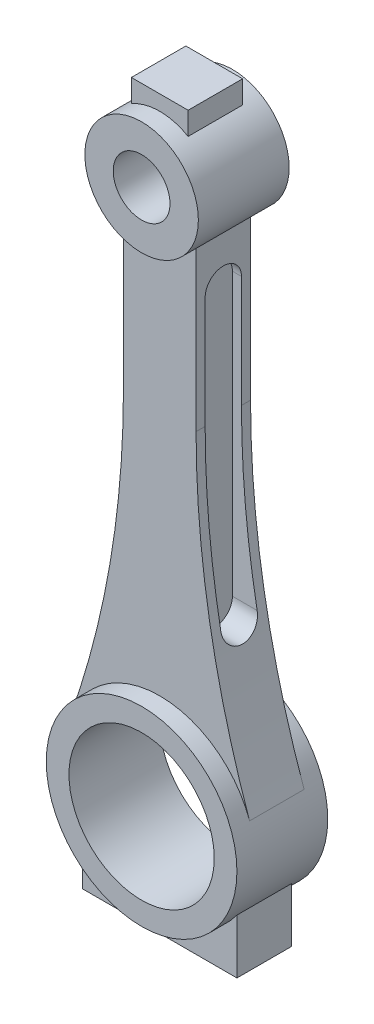
ISO-10303-21;
HEADER;
FILE_DESCRIPTION(('STEP AP214'),'2;1');
FILE_NAME('part.step','',(''),(''),'','','');
FILE_SCHEMA(('AUTOMOTIVE_DESIGN { 1 0 10303 214 1 1 1 1 }'));
ENDSEC;
DATA;
#1=APPLICATION_CONTEXT('core data for automotive mechanical design processes');
#2=APPLICATION_PROTOCOL_DEFINITION('international standard','automotive_design',2000,#1);
#3=PRODUCT_CONTEXT('',#1,'mechanical');
#4=PRODUCT('Part','Part','',(#3));
#5=PRODUCT_RELATED_PRODUCT_CATEGORY('part','',(#4));
#6=PRODUCT_DEFINITION_FORMATION('','',#4);
#7=PRODUCT_DEFINITION_CONTEXT('part definition',#1,'design');
#8=PRODUCT_DEFINITION('design','',#6,#7);
#9=PRODUCT_DEFINITION_SHAPE('','',#8);
#10=(LENGTH_UNIT() NAMED_UNIT(*) SI_UNIT(.MILLI.,.METRE.));
#11=(NAMED_UNIT(*) PLANE_ANGLE_UNIT() SI_UNIT($,.RADIAN.));
#12=(NAMED_UNIT(*) SI_UNIT($,.STERADIAN.) SOLID_ANGLE_UNIT());
#13=UNCERTAINTY_MEASURE_WITH_UNIT(LENGTH_MEASURE(1.E-05),#10,'distance_accuracy_value','');
#14=(GEOMETRIC_REPRESENTATION_CONTEXT(3) GLOBAL_UNCERTAINTY_ASSIGNED_CONTEXT((#13)) GLOBAL_UNIT_ASSIGNED_CONTEXT((#10,
#11,#12)) REPRESENTATION_CONTEXT('',''));
#15=CARTESIAN_POINT('',(0.,0.,0.));
#16=DIRECTION('',(0.,0.,1.));
#17=DIRECTION('',(1.,0.,0.));
#18=AXIS2_PLACEMENT_3D('',#15,#16,#17);
#19=CARTESIAN_POINT('',(212.132819979024,75.3953136438508,6.));
#20=DIRECTION('',(0.,0.,-1.));
#21=DIRECTION('',(-1.,0.,0.));
#22=AXIS2_PLACEMENT_3D('',#19,#20,#21);
#23=CYLINDRICAL_SURFACE('',#22,204.132819979024);
#24=CARTESIAN_POINT('',(11.4544735884215,38.,-4.00000000000001));
#25=CARTESIAN_POINT('',(11.4757515518411,37.8858086335559,-4.00000967356236));
#26=CARTESIAN_POINT('',(11.497127848932,37.7716411229782,-3.9951101211208));
#27=CARTESIAN_POINT('',(11.5399210356049,37.544152772884,-3.97557755361704));
#28=CARTESIAN_POINT('',(11.5613379239584,37.4308319082382,-3.9609448286138));
#29=CARTESIAN_POINT('',(11.6040518019029,37.2058589467753,-3.92203609087538));
#30=CARTESIAN_POINT('',(11.6253488219803,37.0942064124742,-3.89776265395078));
#31=CARTESIAN_POINT('',(11.6676599337569,36.8733657612217,-3.83975872762631));
#32=CARTESIAN_POINT('',(11.688674029376,36.7641776101131,-3.80602836938937));
#33=CARTESIAN_POINT('',(11.7510730473326,36.4413470108117,-3.69089420326938));
#34=CARTESIAN_POINT('',(11.7918289081029,36.2323636826891,-3.59553432969807));
#35=CARTESIAN_POINT('',(11.8702126062764,35.833491871712,-3.37027556179513));
#36=CARTESIAN_POINT('',(11.9078413597511,35.643597793309,-3.24038682968163));
#37=CARTESIAN_POINT('',(11.9784728244352,35.2894796680367,-2.950436910244));
#38=CARTESIAN_POINT('',(12.0115036519544,35.1250988255321,-2.79057453802655));
#39=CARTESIAN_POINT('',(12.0720036427705,34.8256035029566,-2.44449926104123));
#40=CARTESIAN_POINT('',(12.0994724370193,34.6904909648341,-2.25828460915733));
#41=CARTESIAN_POINT('',(12.1473413477104,34.4559602912754,-1.86832249559897));
#42=CARTESIAN_POINT('',(12.1678582991115,34.3559510460777,-1.66494499104501));
#43=CARTESIAN_POINT('',(12.201667760202,34.1915558050773,-1.24372237948287));
#44=CARTESIAN_POINT('',(12.2149615713728,34.1271633917176,-1.02587988675161));
#45=CARTESIAN_POINT('',(12.2336033492388,34.0369591960168,-0.586274812122705));
#46=CARTESIAN_POINT('',(12.2390950212482,34.0104496060439,-0.364661335561854));
#47=CARTESIAN_POINT('',(12.2423732155319,33.9946184843632,0.0799443502249422));
#48=CARTESIAN_POINT('',(12.2401601145853,34.0052951341723,0.302936491499035));
#49=CARTESIAN_POINT('',(12.2281765408432,34.0632127244266,0.741781925824315));
#50=CARTESIAN_POINT('',(12.2184766498272,34.1101121767816,0.957682365575702));
#51=CARTESIAN_POINT('',(12.1919895794175,34.2385791029979,1.37844153266758));
#52=CARTESIAN_POINT('',(12.1752023313576,34.3201469127454,1.58330015300714));
#53=CARTESIAN_POINT('',(12.1350793834177,34.5159552856904,1.977397761575));
#54=CARTESIAN_POINT('',(12.1117098081663,34.6303649264094,2.16654921549123));
#55=CARTESIAN_POINT('',(12.0593260749273,34.8882465100265,2.52297125984127));
#56=CARTESIAN_POINT('',(12.0303117725959,35.0317191961119,2.69024129055298));
#57=CARTESIAN_POINT('',(11.9671383735568,35.3461665633751,3.00114206510914));
#58=CARTESIAN_POINT('',(11.9329025496515,35.5175545383741,3.14433904981939));
#59=CARTESIAN_POINT('',(11.8607975408038,35.8812712267655,3.40006280722765));
#60=CARTESIAN_POINT('',(11.8229268395298,36.0736086840292,3.51257670427656));
#61=CARTESIAN_POINT('',(11.744011046999,36.4777513253325,3.70593438635491));
#62=CARTESIAN_POINT('',(11.7029182624971,36.6898643551292,3.78611370956408));
#63=CARTESIAN_POINT('',(11.619535719839,37.1241795414682,3.90944320644274));
#64=CARTESIAN_POINT('',(11.5772477716993,37.3463667203578,3.95264656840455));
#65=CARTESIAN_POINT('',(11.5215540274852,37.6417241762258,3.98457340087694));
#66=CARTESIAN_POINT('',(11.5080944382148,37.713314753212,3.99036111817268));
#67=CARTESIAN_POINT('',(11.4812368188341,37.8565916807734,3.99806924003837));
#68=CARTESIAN_POINT('',(11.467838723541,37.9282776734255,3.99999606757804));
#69=CARTESIAN_POINT('',(11.4544735884215,38.,3.99999999999999));
#70=B_SPLINE_CURVE_WITH_KNOTS('',3,(#24,#25,#26,#27,#28,#29,#30,#31,#32,#33,#34,#35,#36,#37,#38,
#39,#40,#41,#42,#43,#44,#45,#46,#47,#48,#49,#50,#51,#52,#53,#54,#55,#56,#57,#58,#59,#60,#61,#62,
#63,#64,#65,#66,#67,#68,#69),.UNSPECIFIED.,.F.,.F.,(4,2,2,2,2,2,2,2,2,2,2,2,2,2,2,2,2,2,2,2,2,2,
4),(0.,0.348357600629775,0.69670482029576,1.04495903090802,1.39320841164155,2.08947857427321,
2.78554404346984,3.47714614167073,4.1687941135383,4.84816302804556,5.52740949173436,
6.19397531687089,6.86050854603356,7.52083364695975,8.18116514562694,8.84495910470898,
9.50877004017901,10.1834922182609,10.8584970981523,11.546741507572,12.2339942357506,
12.4531452672714,12.6719314158043),.UNSPECIFIED.);
#71=CARTESIAN_POINT('',(11.4544735884215,38.,-4.00000000000001));
#72=VERTEX_POINT('',#71);
#73=CARTESIAN_POINT('',(11.4544735884215,38.,3.99999999999999));
#74=VERTEX_POINT('',#73);
#75=EDGE_CURVE('E406',#72,#74,#70,.T.);
#76=ORIENTED_EDGE('',*,*,#75,.T.);
#77=CARTESIAN_POINT('',(212.132819979024,75.3953136438508,4.));
#78=DIRECTION('',(0.,0.,-1.));
#79=DIRECTION('',(0.,1.,0.));
#80=AXIS2_PLACEMENT_3D('',#77,#78,#79);
#81=CIRCLE('',#80,204.132819979024);
#82=CARTESIAN_POINT('',(8.,75.3953136438507,4.));
#83=VERTEX_POINT('',#82);
#84=EDGE_CURVE('E265',#74,#83,#81,.T.);
#85=ORIENTED_EDGE('',*,*,#84,.T.);
#86=DIRECTION('',(0.,0.,-1.));
#87=VECTOR('',#86,1.);
#88=CARTESIAN_POINT('',(8.,75.3953136438507,6.));
#89=LINE('',#88,#87);
#90=CARTESIAN_POINT('',(8.,75.3953136438507,6.));
#91=VERTEX_POINT('',#90);
#92=EDGE_CURVE('E386',#91,#83,#89,.T.);
#93=ORIENTED_EDGE('',*,*,#92,.F.);
#94=CARTESIAN_POINT('',(212.132819979024,75.3953136438508,6.));
#95=DIRECTION('',(0.,0.,1.));
#96=DIRECTION('',(1.,0.,0.));
#97=AXIS2_PLACEMENT_3D('',#94,#95,#96);
#98=CIRCLE('',#97,204.132819979024);
#99=CARTESIAN_POINT('',(19.7873824881444,7.03274443356765,6.));
#100=VERTEX_POINT('',#99);
#101=EDGE_CURVE('E341',#91,#100,#98,.T.);
#102=ORIENTED_EDGE('',*,*,#101,.T.);
#103=DIRECTION('',(0.,0.,-1.));
#104=VECTOR('',#103,1.);
#105=CARTESIAN_POINT('',(19.7873824881444,7.03274443356765,6.));
#106=LINE('',#105,#104);
#107=CARTESIAN_POINT('',(19.7873824881444,7.03274443356765,-6.));
#108=VERTEX_POINT('',#107);
#109=EDGE_CURVE('E357',#100,#108,#106,.T.);
#110=ORIENTED_EDGE('',*,*,#109,.T.);
#111=CARTESIAN_POINT('',(212.132819979024,75.3953136438508,-6.));
#112=DIRECTION('',(0.,0.,1.));
#113=DIRECTION('',(1.,0.,0.));
#114=AXIS2_PLACEMENT_3D('',#111,#112,#113);
#115=CIRCLE('',#114,204.132819979024);
#116=CARTESIAN_POINT('',(8.,75.3953136438507,-6.));
#117=VERTEX_POINT('',#116);
#118=EDGE_CURVE('E338',#117,#108,#115,.T.);
#119=ORIENTED_EDGE('',*,*,#118,.F.);
#120=CARTESIAN_POINT('',(8.,75.3953136438507,-4.));
#121=VERTEX_POINT('',#120);
#122=EDGE_CURVE('E389',#121,#117,#89,.T.);
#123=ORIENTED_EDGE('',*,*,#122,.F.);
#124=CARTESIAN_POINT('',(212.132819979024,75.3953136438508,-4.00000000000001));
#125=DIRECTION('',(0.,0.,1.));
#126=DIRECTION('',(0.,-1.,0.));
#127=AXIS2_PLACEMENT_3D('',#124,#125,#126);
#128=CIRCLE('',#127,204.132819979024);
#129=EDGE_CURVE('E67',#121,#72,#128,.T.);
#130=ORIENTED_EDGE('',*,*,#129,.T.);
#131=EDGE_LOOP('',(#76,#85,#93,#102,#110,#119,#123,#130));
#132=FACE_BOUND('',#131,.T.);
#133=ADVANCED_FACE('F44',(#132),#23,.F.);
#134=CARTESIAN_POINT('',(8.00000000000002,0.,6.));
#135=DIRECTION('',(-1.,0.,0.));
#136=DIRECTION('',(0.,-1.,0.));
#137=AXIS2_PLACEMENT_3D('',#134,#135,#136);
#138=PLANE('',#137);
#139=DIRECTION('',(0.,-1.,0.));
#140=VECTOR('',#139,1.);
#141=CARTESIAN_POINT('',(8.00000000000002,0.,3.99999999999999));
#142=LINE('',#141,#140);
#143=CARTESIAN_POINT('',(8.00000000000001,100.,4.));
#144=VERTEX_POINT('',#143);
#145=EDGE_CURVE('E407',#144,#83,#142,.T.);
#146=ORIENTED_EDGE('',*,*,#145,.F.);
#147=CARTESIAN_POINT('',(8.,100.,0.));
#148=DIRECTION('',(-1.,0.,0.));
#149=DIRECTION('',(0.,-1.,0.));
#150=AXIS2_PLACEMENT_3D('',#147,#148,#149);
#151=CIRCLE('',#150,4.);
#152=CARTESIAN_POINT('',(8.00000000000001,100.,-4.));
#153=VERTEX_POINT('',#152);
#154=EDGE_CURVE('E408',#153,#144,#151,.F.);
#155=ORIENTED_EDGE('',*,*,#154,.F.);
#156=DIRECTION('',(0.,1.,0.));
#157=VECTOR('',#156,1.);
#158=CARTESIAN_POINT('',(8.00000000000002,0.,-4.00000000000001));
#159=LINE('',#158,#157);
#160=EDGE_CURVE('E399',#121,#153,#159,.T.);
#161=ORIENTED_EDGE('',*,*,#160,.F.);
#162=ORIENTED_EDGE('',*,*,#122,.T.);
#163=DIRECTION('',(0.,1.,0.));
#164=VECTOR('',#163,1.);
#165=CARTESIAN_POINT('',(8.00000000000002,0.,-6.));
#166=LINE('',#165,#164);
#167=CARTESIAN_POINT('',(8.,110.395313643851,-6.));
#168=VERTEX_POINT('',#167);
#169=EDGE_CURVE('E363',#117,#168,#166,.T.);
#170=ORIENTED_EDGE('',*,*,#169,.T.);
#171=DIRECTION('',(0.,0.,-1.));
#172=VECTOR('',#171,1.);
#173=CARTESIAN_POINT('',(8.,110.395313643851,6.));
#174=LINE('',#173,#172);
#175=CARTESIAN_POINT('',(8.,110.395313643851,6.));
#176=VERTEX_POINT('',#175);
#177=EDGE_CURVE('E387',#176,#168,#174,.T.);
#178=ORIENTED_EDGE('',*,*,#177,.F.);
#179=DIRECTION('',(0.,1.,0.));
#180=VECTOR('',#179,1.);
#181=CARTESIAN_POINT('',(8.00000000000002,0.,6.));
#182=LINE('',#181,#180);
#183=EDGE_CURVE('E343',#91,#176,#182,.T.);
#184=ORIENTED_EDGE('',*,*,#183,.F.);
#185=ORIENTED_EDGE('',*,*,#92,.T.);
#186=EDGE_LOOP('',(#146,#155,#161,#162,#170,#178,#184,#185));
#187=FACE_BOUND('',#186,.T.);
#188=ADVANCED_FACE('F536',(#187),#138,.F.);
#189=CARTESIAN_POINT('',(0.,120.,10.));
#190=DIRECTION('',(0.,0.,-1.));
#191=DIRECTION('',(-1.,0.,0.));
#192=AXIS2_PLACEMENT_3D('',#189,#190,#191);
#193=CYLINDRICAL_SURFACE('',#192,6.25);
#194=CARTESIAN_POINT('',(0.,120.,10.));
#195=DIRECTION('',(0.,0.,1.));
#196=DIRECTION('',(1.,0.,0.));
#197=AXIS2_PLACEMENT_3D('',#194,#195,#196);
#198=CIRCLE('',#197,6.25);
#199=CARTESIAN_POINT('',(6.25,120.,10.));
#200=VERTEX_POINT('',#199);
#201=EDGE_CURVE('E392',#200,#200,#198,.T.);
#202=ORIENTED_EDGE('',*,*,#201,.T.);
#203=EDGE_LOOP('',(#202));
#204=FACE_BOUND('',#203,.T.);
#205=CARTESIAN_POINT('',(0.,120.,-10.));
#206=DIRECTION('',(0.,0.,1.));
#207=DIRECTION('',(1.,0.,0.));
#208=AXIS2_PLACEMENT_3D('',#205,#206,#207);
#209=CIRCLE('',#208,6.25);
#210=CARTESIAN_POINT('',(6.25,120.,-10.));
#211=VERTEX_POINT('',#210);
#212=EDGE_CURVE('E394',#211,#211,#209,.T.);
#213=ORIENTED_EDGE('',*,*,#212,.F.);
#214=EDGE_LOOP('',(#213));
#215=FACE_BOUND('',#214,.T.);
#216=ADVANCED_FACE('F50',(#204,#215),#193,.F.);
#217=CARTESIAN_POINT('',(0.,120.,10.));
#218=DIRECTION('',(0.,0.,-1.));
#219=DIRECTION('',(-1.,0.,0.));
#220=AXIS2_PLACEMENT_3D('',#217,#218,#219);
#221=CYLINDRICAL_SURFACE('',#220,12.5);
#222=DIRECTION('',(0.,0.,-1.));
#223=VECTOR('',#222,1.);
#224=CARTESIAN_POINT('',(6.25,130.825317547305,6.));
#225=LINE('',#224,#223);
#226=CARTESIAN_POINT('',(6.25,130.825317547305,6.));
#227=VERTEX_POINT('',#226);
#228=CARTESIAN_POINT('',(6.25,130.825317547305,-6.));
#229=VERTEX_POINT('',#228);
#230=EDGE_CURVE('E324',#227,#229,#225,.T.);
#231=ORIENTED_EDGE('',*,*,#230,.F.);
#232=CARTESIAN_POINT('',(0.,120.,6.));
#233=DIRECTION('',(0.,0.,1.));
#234=DIRECTION('',(1.,0.,0.));
#235=AXIS2_PLACEMENT_3D('',#232,#233,#234);
#236=CIRCLE('',#235,12.5);
#237=CARTESIAN_POINT('',(-6.25,130.825317547305,6.));
#238=VERTEX_POINT('',#237);
#239=EDGE_CURVE('E297',#227,#238,#236,.T.);
#240=ORIENTED_EDGE('',*,*,#239,.T.);
#241=DIRECTION('',(0.,0.,-1.));
#242=VECTOR('',#241,1.);
#243=CARTESIAN_POINT('',(-6.25,130.825317547305,6.));
#244=LINE('',#243,#242);
#245=CARTESIAN_POINT('',(-6.25,130.825317547305,-6.));
#246=VERTEX_POINT('',#245);
#247=EDGE_CURVE('E310',#238,#246,#244,.T.);
#248=ORIENTED_EDGE('',*,*,#247,.T.);
#249=CARTESIAN_POINT('',(0.,120.,-6.));
#250=DIRECTION('',(0.,0.,1.));
#251=DIRECTION('',(1.,0.,0.));
#252=AXIS2_PLACEMENT_3D('',#249,#250,#251);
#253=CIRCLE('',#252,12.5);
#254=EDGE_CURVE('E299',#229,#246,#253,.T.);
#255=ORIENTED_EDGE('',*,*,#254,.F.);
#256=EDGE_LOOP('',(#231,#240,#248,#255));
#257=FACE_BOUND('',#256,.T.);
#258=DIRECTION('',(0.,0.,-1.));
#259=VECTOR('',#258,1.);
#260=CARTESIAN_POINT('',(-7.99999999999999,110.395313643851,6.));
#261=LINE('',#260,#259);
#262=CARTESIAN_POINT('',(-7.99999999999999,110.395313643851,6.));
#263=VERTEX_POINT('',#262);
#264=CARTESIAN_POINT('',(-7.99999999999999,110.395313643851,-6.));
#265=VERTEX_POINT('',#264);
#266=EDGE_CURVE('E382',#263,#265,#261,.T.);
#267=ORIENTED_EDGE('',*,*,#266,.F.);
#268=CARTESIAN_POINT('',(0.,120.,6.));
#269=DIRECTION('',(0.,0.,1.));
#270=DIRECTION('',(1.,0.,0.));
#271=AXIS2_PLACEMENT_3D('',#268,#269,#270);
#272=CIRCLE('',#271,12.5);
#273=EDGE_CURVE('E346',#263,#176,#272,.T.);
#274=ORIENTED_EDGE('',*,*,#273,.T.);
#275=ORIENTED_EDGE('',*,*,#177,.T.);
#276=CARTESIAN_POINT('',(0.,120.,-6.));
#277=DIRECTION('',(0.,0.,1.));
#278=DIRECTION('',(1.,0.,0.));
#279=AXIS2_PLACEMENT_3D('',#276,#277,#278);
#280=CIRCLE('',#279,12.5);
#281=EDGE_CURVE('E365',#265,#168,#280,.T.);
#282=ORIENTED_EDGE('',*,*,#281,.F.);
#283=EDGE_LOOP('',(#267,#274,#275,#282));
#284=FACE_BOUND('',#283,.T.);
#285=CARTESIAN_POINT('',(0.,120.,10.));
#286=DIRECTION('',(0.,0.,1.));
#287=DIRECTION('',(1.,0.,0.));
#288=AXIS2_PLACEMENT_3D('',#285,#286,#287);
#289=CIRCLE('',#288,12.5);
#290=CARTESIAN_POINT('',(12.5,120.,10.));
#291=VERTEX_POINT('',#290);
#292=EDGE_CURVE('E396',#291,#291,#289,.T.);
#293=ORIENTED_EDGE('',*,*,#292,.F.);
#294=EDGE_LOOP('',(#293));
#295=FACE_BOUND('',#294,.T.);
#296=CARTESIAN_POINT('',(0.,120.,-10.));
#297=DIRECTION('',(0.,0.,1.));
#298=DIRECTION('',(1.,0.,0.));
#299=AXIS2_PLACEMENT_3D('',#296,#297,#298);
#300=CIRCLE('',#299,12.5);
#301=CARTESIAN_POINT('',(12.5,120.,-10.));
#302=VERTEX_POINT('',#301);
#303=EDGE_CURVE('E400',#302,#302,#300,.T.);
#304=ORIENTED_EDGE('',*,*,#303,.T.);
#305=EDGE_LOOP('',(#304));
#306=FACE_BOUND('',#305,.T.);
#307=ADVANCED_FACE('F567',(#257,#284,#295,#306),#221,.T.);
#308=CARTESIAN_POINT('',(0.,0.,10.));
#309=DIRECTION('',(0.,0.,1.));
#310=DIRECTION('',(1.,0.,0.));
#311=AXIS2_PLACEMENT_3D('',#308,#309,#310);
#312=PLANE('',#311);
#313=ORIENTED_EDGE('',*,*,#201,.F.);
#314=EDGE_LOOP('',(#313));
#315=FACE_BOUND('',#314,.T.);
#316=ORIENTED_EDGE('',*,*,#292,.T.);
#317=EDGE_LOOP('',(#316));
#318=FACE_BOUND('',#317,.T.);
#319=ADVANCED_FACE('F648',(#315,#318),#312,.T.);
#320=CARTESIAN_POINT('',(0.,0.,-10.));
#321=DIRECTION('',(0.,0.,1.));
#322=DIRECTION('',(1.,0.,0.));
#323=AXIS2_PLACEMENT_3D('',#320,#321,#322);
#324=PLANE('',#323);
#325=ORIENTED_EDGE('',*,*,#212,.T.);
#326=EDGE_LOOP('',(#325));
#327=FACE_BOUND('',#326,.T.);
#328=ORIENTED_EDGE('',*,*,#303,.F.);
#329=EDGE_LOOP('',(#328));
#330=FACE_BOUND('',#329,.T.);
#331=ADVANCED_FACE('F620',(#327,#330),#324,.F.);
#332=CARTESIAN_POINT('',(-7.99999999999999,0.,6.));
#333=DIRECTION('',(-1.,0.,0.));
#334=DIRECTION('',(0.,0.,1.));
#335=AXIS2_PLACEMENT_3D('',#332,#333,#334);
#336=PLANE('',#335);
#337=DIRECTION('',(0.,-1.,0.));
#338=VECTOR('',#337,1.);
#339=CARTESIAN_POINT('',(-7.99999999999999,0.,-4.00000000000001));
#340=LINE('',#339,#338);
#341=CARTESIAN_POINT('',(-8.,100.,-4.));
#342=VERTEX_POINT('',#341);
#343=CARTESIAN_POINT('',(-8.00000000000001,75.3953136438507,-4.00000000000001));
#344=VERTEX_POINT('',#343);
#345=EDGE_CURVE('E239',#342,#344,#340,.T.);
#346=ORIENTED_EDGE('',*,*,#345,.F.);
#347=CARTESIAN_POINT('',(-7.99999999999999,100.,0.));
#348=DIRECTION('',(-1.,0.,0.));
#349=DIRECTION('',(0.,0.,1.));
#350=AXIS2_PLACEMENT_3D('',#347,#348,#349);
#351=CIRCLE('',#350,4.);
#352=CARTESIAN_POINT('',(-8.,100.,4.));
#353=VERTEX_POINT('',#352);
#354=EDGE_CURVE('E11',#353,#342,#351,.T.);
#355=ORIENTED_EDGE('',*,*,#354,.F.);
#356=DIRECTION('',(0.,1.,0.));
#357=VECTOR('',#356,1.);
#358=CARTESIAN_POINT('',(-7.99999999999999,0.,3.99999999999999));
#359=LINE('',#358,#357);
#360=CARTESIAN_POINT('',(-8.00000000000001,75.3953136438507,4.));
#361=VERTEX_POINT('',#360);
#362=EDGE_CURVE('E216',#361,#353,#359,.T.);
#363=ORIENTED_EDGE('',*,*,#362,.F.);
#364=DIRECTION('',(0.,0.,-1.));
#365=VECTOR('',#364,1.);
#366=CARTESIAN_POINT('',(-7.99999999999999,75.3953136438507,6.));
#367=LINE('',#366,#365);
#368=CARTESIAN_POINT('',(-7.99999999999999,75.3953136438507,6.));
#369=VERTEX_POINT('',#368);
#370=EDGE_CURVE('E379',#369,#361,#367,.T.);
#371=ORIENTED_EDGE('',*,*,#370,.F.);
#372=DIRECTION('',(0.,1.,0.));
#373=VECTOR('',#372,1.);
#374=CARTESIAN_POINT('',(-7.99999999999999,0.,6.));
#375=LINE('',#374,#373);
#376=EDGE_CURVE('E348',#369,#263,#375,.T.);
#377=ORIENTED_EDGE('',*,*,#376,.T.);
#378=ORIENTED_EDGE('',*,*,#266,.T.);
#379=DIRECTION('',(0.,1.,0.));
#380=VECTOR('',#379,1.);
#381=CARTESIAN_POINT('',(-7.99999999999999,0.,-6.));
#382=LINE('',#381,#380);
#383=CARTESIAN_POINT('',(-7.99999999999999,75.3953136438507,-6.));
#384=VERTEX_POINT('',#383);
#385=EDGE_CURVE('E370',#384,#265,#382,.T.);
#386=ORIENTED_EDGE('',*,*,#385,.F.);
#387=EDGE_CURVE('E377',#344,#384,#367,.T.);
#388=ORIENTED_EDGE('',*,*,#387,.F.);
#389=EDGE_LOOP('',(#346,#355,#363,#371,#377,#378,#386,#388));
#390=FACE_BOUND('',#389,.T.);
#391=ADVANCED_FACE('F507',(#390),#336,.T.);
#392=CARTESIAN_POINT('',(-212.132819979024,75.3953136438507,6.));
#393=DIRECTION('',(0.,0.,-1.));
#394=DIRECTION('',(-1.,0.,0.));
#395=AXIS2_PLACEMENT_3D('',#392,#393,#394);
#396=CYLINDRICAL_SURFACE('',#395,204.132819979024);
#397=CARTESIAN_POINT('',(-11.4544735884215,38.,3.99999999999999));
#398=CARTESIAN_POINT('',(-11.4757515518411,37.8858086335559,4.00000967356234));
#399=CARTESIAN_POINT('',(-11.497127848932,37.7716411229782,3.99511012112078));
#400=CARTESIAN_POINT('',(-11.5399210356049,37.544152772884,3.97557755361703));
#401=CARTESIAN_POINT('',(-11.5613379239584,37.4308319082382,3.96094482861378));
#402=CARTESIAN_POINT('',(-11.6040518019029,37.2058589467753,3.92203609087537));
#403=CARTESIAN_POINT('',(-11.6253488219802,37.0942064124742,3.89776265395076));
#404=CARTESIAN_POINT('',(-11.6676599337569,36.8733657612217,3.83975872762629));
#405=CARTESIAN_POINT('',(-11.6886740293759,36.7641776101131,3.80602836938935));
#406=CARTESIAN_POINT('',(-11.7510730473326,36.4413470108117,3.69089420326937));
#407=CARTESIAN_POINT('',(-11.7918289081029,36.2323636826891,3.59553432969806));
#408=CARTESIAN_POINT('',(-11.8702126062764,35.833491871712,3.37027556179512));
#409=CARTESIAN_POINT('',(-11.9078413597511,35.643597793309,3.24038682968162));
#410=CARTESIAN_POINT('',(-11.9784728244352,35.2894796680367,2.95043691024399));
#411=CARTESIAN_POINT('',(-12.0115036519544,35.1250988255321,2.79057453802654));
#412=CARTESIAN_POINT('',(-12.0720036427705,34.8256035029566,2.44449926104123));
#413=CARTESIAN_POINT('',(-12.0994724370193,34.6904909648341,2.25828460915732));
#414=CARTESIAN_POINT('',(-12.1473413477104,34.4559602912754,1.86832249559895));
#415=CARTESIAN_POINT('',(-12.1678582991115,34.3559510460777,1.66494499104499));
#416=CARTESIAN_POINT('',(-12.201667760202,34.1915558050773,1.24372237948286));
#417=CARTESIAN_POINT('',(-12.2149615713728,34.1271633917176,1.02587988675159));
#418=CARTESIAN_POINT('',(-12.2336033492388,34.0369591960168,0.586274812122689));
#419=CARTESIAN_POINT('',(-12.2390950212481,34.0104496060439,0.364661335561839));
#420=CARTESIAN_POINT('',(-12.2423732155318,33.9946184843632,-0.0799443502249572));
#421=CARTESIAN_POINT('',(-12.2401601145853,34.0052951341723,-0.30293649149905));
#422=CARTESIAN_POINT('',(-12.2281765408432,34.0632127244266,-0.74178192582433));
#423=CARTESIAN_POINT('',(-12.2184766498272,34.1101121767816,-0.957682365575717));
#424=CARTESIAN_POINT('',(-12.1919895794175,34.2385791029979,-1.3784415326676));
#425=CARTESIAN_POINT('',(-12.1752023313576,34.3201469127454,-1.58330015300716));
#426=CARTESIAN_POINT('',(-12.1350793834177,34.5159552856904,-1.97739776157502));
#427=CARTESIAN_POINT('',(-12.1117098081663,34.6303649264094,-2.16654921549125));
#428=CARTESIAN_POINT('',(-12.0593260749273,34.8882465100265,-2.52297125984129));
#429=CARTESIAN_POINT('',(-12.0303117725959,35.0317191961119,-2.690241290553));
#430=CARTESIAN_POINT('',(-11.9671383735568,35.3461665633751,-3.00114206510916));
#431=CARTESIAN_POINT('',(-11.9329025496515,35.5175545383741,-3.14433904981941));
#432=CARTESIAN_POINT('',(-11.8607975408038,35.8812712267655,-3.40006280722766));
#433=CARTESIAN_POINT('',(-11.8229268395298,36.0736086840292,-3.51257670427658));
#434=CARTESIAN_POINT('',(-11.744011046999,36.4777513253325,-3.70593438635493));
#435=CARTESIAN_POINT('',(-11.7029182624971,36.6898643551292,-3.78611370956409));
#436=CARTESIAN_POINT('',(-11.6195357198389,37.1241795414682,-3.90944320644275));
#437=CARTESIAN_POINT('',(-11.5772477716993,37.3463667203578,-3.95264656840456));
#438=CARTESIAN_POINT('',(-11.5215540274853,37.6417241762258,-3.98457340087696));
#439=CARTESIAN_POINT('',(-11.5080944382149,37.713314753212,-3.9903611181727));
#440=CARTESIAN_POINT('',(-11.4812368188341,37.8565916807733,-3.99806924003838));
#441=CARTESIAN_POINT('',(-11.467838723541,37.9282776734255,-3.99999606757806));
#442=CARTESIAN_POINT('',(-11.4544735884215,38.,-4.00000000000001));
#443=B_SPLINE_CURVE_WITH_KNOTS('',3,(#397,#398,#399,#400,#401,#402,#403,#404,#405,#406,#407,
#408,#409,#410,#411,#412,#413,#414,#415,#416,#417,#418,#419,#420,#421,#422,#423,#424,#425,#426,
#427,#428,#429,#430,#431,#432,#433,#434,#435,#436,#437,#438,#439,#440,#441,#442),.UNSPECIFIED.,
.F.,.F.,(4,2,2,2,2,2,2,2,2,2,2,2,2,2,2,2,2,2,2,2,2,2,4),(0.,0.348357600629778,0.696704820295753,
1.044959030908,1.39320841164154,2.0894785742732,2.78554404346983,3.47714614167072,
4.1687941135383,4.84816302804556,5.52740949173436,6.19397531687089,6.86050854603355,
7.52083364695974,8.18116514562693,8.84495910470897,9.508770040179,10.1834922182609,
10.8584970981523,11.546741507572,12.2339942357505,12.4531452672714,12.6719314158043),.UNSPECIFIED.);
#444=CARTESIAN_POINT('',(-11.4544735884215,38.,3.99999999999999));
#445=VERTEX_POINT('',#444);
#446=CARTESIAN_POINT('',(-11.4544735884215,38.,-4.00000000000001));
#447=VERTEX_POINT('',#446);
#448=EDGE_CURVE('E509',#445,#447,#443,.T.);
#449=ORIENTED_EDGE('',*,*,#448,.T.);
#450=CARTESIAN_POINT('',(-212.132819979024,75.3953136438507,-4.00000000000001));
#451=DIRECTION('',(0.,0.,-1.));
#452=DIRECTION('',(0.,1.,0.));
#453=AXIS2_PLACEMENT_3D('',#450,#451,#452);
#454=CIRCLE('',#453,204.132819979024);
#455=EDGE_CURVE('E52',#447,#344,#454,.F.);
#456=ORIENTED_EDGE('',*,*,#455,.T.);
#457=ORIENTED_EDGE('',*,*,#387,.T.);
#458=CARTESIAN_POINT('',(-212.132819979024,75.3953136438507,-6.));
#459=DIRECTION('',(0.,0.,1.));
#460=DIRECTION('',(1.,0.,0.));
#461=AXIS2_PLACEMENT_3D('',#458,#459,#460);
#462=CIRCLE('',#461,204.132819979024);
#463=CARTESIAN_POINT('',(-19.7873824881444,7.03274443356764,-6.));
#464=VERTEX_POINT('',#463);
#465=EDGE_CURVE('E367',#384,#464,#462,.F.);
#466=ORIENTED_EDGE('',*,*,#465,.T.);
#467=DIRECTION('',(0.,0.,-1.));
#468=VECTOR('',#467,1.);
#469=CARTESIAN_POINT('',(-19.7873824881444,7.03274443356764,6.));
#470=LINE('',#469,#468);
#471=CARTESIAN_POINT('',(-19.7873824881444,7.03274443356764,6.));
#472=VERTEX_POINT('',#471);
#473=EDGE_CURVE('E380',#472,#464,#470,.T.);
#474=ORIENTED_EDGE('',*,*,#473,.F.);
#475=CARTESIAN_POINT('',(-212.132819979024,75.3953136438507,6.));
#476=DIRECTION('',(0.,0.,1.));
#477=DIRECTION('',(1.,0.,0.));
#478=AXIS2_PLACEMENT_3D('',#475,#476,#477);
#479=CIRCLE('',#478,204.132819979024);
#480=EDGE_CURVE('E352',#369,#472,#479,.F.);
#481=ORIENTED_EDGE('',*,*,#480,.F.);
#482=ORIENTED_EDGE('',*,*,#370,.T.);
#483=CARTESIAN_POINT('',(-212.132819979024,75.3953136438507,4.));
#484=DIRECTION('',(0.,0.,1.));
#485=DIRECTION('',(0.,-1.,0.));
#486=AXIS2_PLACEMENT_3D('',#483,#484,#485);
#487=CIRCLE('',#486,204.132819979024);
#488=EDGE_CURVE('E420',#361,#445,#487,.F.);
#489=ORIENTED_EDGE('',*,*,#488,.T.);
#490=EDGE_LOOP('',(#449,#456,#457,#466,#474,#481,#482,#489));
#491=FACE_BOUND('',#490,.T.);
#492=ADVANCED_FACE('F498',(#491),#396,.F.);
#493=CARTESIAN_POINT('',(0.,0.,6.));
#494=DIRECTION('',(0.,0.,1.));
#495=DIRECTION('',(1.,0.,0.));
#496=AXIS2_PLACEMENT_3D('',#493,#494,#495);
#497=PLANE('',#496);
#498=ORIENTED_EDGE('',*,*,#101,.F.);
#499=ORIENTED_EDGE('',*,*,#183,.T.);
#500=ORIENTED_EDGE('',*,*,#273,.F.);
#501=ORIENTED_EDGE('',*,*,#376,.F.);
#502=ORIENTED_EDGE('',*,*,#480,.T.);
#503=CARTESIAN_POINT('',(0.,0.,6.));
#504=DIRECTION('',(0.,0.,1.));
#505=DIRECTION('',(1.,0.,0.));
#506=AXIS2_PLACEMENT_3D('',#503,#504,#505);
#507=CIRCLE('',#506,21.);
#508=EDGE_CURVE('E356',#100,#472,#507,.T.);
#509=ORIENTED_EDGE('',*,*,#508,.F.);
#510=EDGE_LOOP('',(#498,#499,#500,#501,#502,#509));
#511=FACE_BOUND('',#510,.T.);
#512=ADVANCED_FACE('F500',(#511),#497,.T.);
#513=CARTESIAN_POINT('',(0.,0.,-6.));
#514=DIRECTION('',(0.,0.,1.));
#515=DIRECTION('',(1.,0.,0.));
#516=AXIS2_PLACEMENT_3D('',#513,#514,#515);
#517=PLANE('',#516);
#518=ORIENTED_EDGE('',*,*,#118,.T.);
#519=CARTESIAN_POINT('',(0.,0.,-6.));
#520=DIRECTION('',(0.,0.,1.));
#521=DIRECTION('',(1.,0.,0.));
#522=AXIS2_PLACEMENT_3D('',#519,#520,#521);
#523=CIRCLE('',#522,21.);
#524=EDGE_CURVE('E344',#108,#464,#523,.T.);
#525=ORIENTED_EDGE('',*,*,#524,.T.);
#526=ORIENTED_EDGE('',*,*,#465,.F.);
#527=ORIENTED_EDGE('',*,*,#385,.T.);
#528=ORIENTED_EDGE('',*,*,#281,.T.);
#529=ORIENTED_EDGE('',*,*,#169,.F.);
#530=EDGE_LOOP('',(#518,#525,#526,#527,#528,#529));
#531=FACE_BOUND('',#530,.T.);
#532=ADVANCED_FACE('F494',(#531),#517,.F.);
#533=CARTESIAN_POINT('',(0.,0.,10.));
#534=DIRECTION('',(0.,0.,-1.));
#535=DIRECTION('',(-1.,0.,0.));
#536=AXIS2_PLACEMENT_3D('',#533,#534,#535);
#537=CYLINDRICAL_SURFACE('',#536,16.);
#538=CARTESIAN_POINT('',(0.,0.,10.));
#539=DIRECTION('',(0.,0.,1.));
#540=DIRECTION('',(1.,0.,0.));
#541=AXIS2_PLACEMENT_3D('',#538,#539,#540);
#542=CIRCLE('',#541,16.);
#543=CARTESIAN_POINT('',(16.,0.,10.));
#544=VERTEX_POINT('',#543);
#545=EDGE_CURVE('E328',#544,#544,#542,.T.);
#546=ORIENTED_EDGE('',*,*,#545,.T.);
#547=EDGE_LOOP('',(#546));
#548=FACE_BOUND('',#547,.T.);
#549=CARTESIAN_POINT('',(0.,0.,-10.));
#550=DIRECTION('',(0.,0.,1.));
#551=DIRECTION('',(1.,0.,0.));
#552=AXIS2_PLACEMENT_3D('',#549,#550,#551);
#553=CIRCLE('',#552,16.);
#554=CARTESIAN_POINT('',(16.,0.,-10.));
#555=VERTEX_POINT('',#554);
#556=EDGE_CURVE('E327',#555,#555,#553,.T.);
#557=ORIENTED_EDGE('',*,*,#556,.F.);
#558=EDGE_LOOP('',(#557));
#559=FACE_BOUND('',#558,.T.);
#560=ADVANCED_FACE('F491',(#548,#559),#537,.F.);
#561=CARTESIAN_POINT('',(0.,0.,10.));
#562=DIRECTION('',(0.,0.,-1.));
#563=DIRECTION('',(-1.,0.,0.));
#564=AXIS2_PLACEMENT_3D('',#561,#562,#563);
#565=CYLINDRICAL_SURFACE('',#564,21.);
#566=DIRECTION('',(0.,0.,-1.));
#567=VECTOR('',#566,1.);
#568=CARTESIAN_POINT('',(-17.,-12.328828005938,6.));
#569=LINE('',#568,#567);
#570=CARTESIAN_POINT('',(-17.,-12.328828005938,6.));
#571=VERTEX_POINT('',#570);
#572=CARTESIAN_POINT('',(-17.,-12.328828005938,-6.));
#573=VERTEX_POINT('',#572);
#574=EDGE_CURVE('E294',#571,#573,#569,.T.);
#575=ORIENTED_EDGE('',*,*,#574,.F.);
#576=CARTESIAN_POINT('',(0.,0.,6.));
#577=DIRECTION('',(0.,0.,1.));
#578=DIRECTION('',(1.,0.,0.));
#579=AXIS2_PLACEMENT_3D('',#576,#577,#578);
#580=CIRCLE('',#579,21.);
#581=CARTESIAN_POINT('',(17.,-12.328828005938,6.));
#582=VERTEX_POINT('',#581);
#583=EDGE_CURVE('E266',#571,#582,#580,.T.);
#584=ORIENTED_EDGE('',*,*,#583,.T.);
#585=DIRECTION('',(0.,0.,-1.));
#586=VECTOR('',#585,1.);
#587=CARTESIAN_POINT('',(17.,-12.328828005938,6.));
#588=LINE('',#587,#586);
#589=CARTESIAN_POINT('',(17.,-12.328828005938,-6.));
#590=VERTEX_POINT('',#589);
#591=EDGE_CURVE('E279',#582,#590,#588,.T.);
#592=ORIENTED_EDGE('',*,*,#591,.T.);
#593=CARTESIAN_POINT('',(0.,0.,-6.));
#594=DIRECTION('',(0.,0.,1.));
#595=DIRECTION('',(1.,0.,0.));
#596=AXIS2_PLACEMENT_3D('',#593,#594,#595);
#597=CIRCLE('',#596,21.);
#598=EDGE_CURVE('E264',#573,#590,#597,.T.);
#599=ORIENTED_EDGE('',*,*,#598,.F.);
#600=EDGE_LOOP('',(#575,#584,#592,#599));
#601=FACE_BOUND('',#600,.T.);
#602=ORIENTED_EDGE('',*,*,#508,.T.);
#603=ORIENTED_EDGE('',*,*,#473,.T.);
#604=ORIENTED_EDGE('',*,*,#524,.F.);
#605=ORIENTED_EDGE('',*,*,#109,.F.);
#606=EDGE_LOOP('',(#602,#603,#604,#605));
#607=FACE_BOUND('',#606,.T.);
#608=CARTESIAN_POINT('',(0.,0.,10.));
#609=DIRECTION('',(0.,0.,1.));
#610=DIRECTION('',(1.,0.,0.));
#611=AXIS2_PLACEMENT_3D('',#608,#609,#610);
#612=CIRCLE('',#611,21.);
#613=CARTESIAN_POINT('',(21.,0.,10.));
#614=VERTEX_POINT('',#613);
#615=EDGE_CURVE('E335',#614,#614,#612,.T.);
#616=ORIENTED_EDGE('',*,*,#615,.F.);
#617=EDGE_LOOP('',(#616));
#618=FACE_BOUND('',#617,.T.);
#619=CARTESIAN_POINT('',(0.,0.,-10.));
#620=DIRECTION('',(0.,0.,1.));
#621=DIRECTION('',(1.,0.,0.));
#622=AXIS2_PLACEMENT_3D('',#619,#620,#621);
#623=CIRCLE('',#622,21.);
#624=CARTESIAN_POINT('',(21.,0.,-10.));
#625=VERTEX_POINT('',#624);
#626=EDGE_CURVE('E334',#625,#625,#623,.T.);
#627=ORIENTED_EDGE('',*,*,#626,.T.);
#628=EDGE_LOOP('',(#627));
#629=FACE_BOUND('',#628,.T.);
#630=ADVANCED_FACE('F482',(#601,#607,#618,#629),#565,.T.);
#631=CARTESIAN_POINT('',(0.,0.,10.));
#632=DIRECTION('',(0.,0.,1.));
#633=DIRECTION('',(1.,0.,0.));
#634=AXIS2_PLACEMENT_3D('',#631,#632,#633);
#635=PLANE('',#634);
#636=ORIENTED_EDGE('',*,*,#545,.F.);
#637=EDGE_LOOP('',(#636));
#638=FACE_BOUND('',#637,.T.);
#639=ORIENTED_EDGE('',*,*,#615,.T.);
#640=EDGE_LOOP('',(#639));
#641=FACE_BOUND('',#640,.T.);
#642=ADVANCED_FACE('F481',(#638,#641),#635,.T.);
#643=CARTESIAN_POINT('',(0.,0.,-10.));
#644=DIRECTION('',(0.,0.,1.));
#645=DIRECTION('',(1.,0.,0.));
#646=AXIS2_PLACEMENT_3D('',#643,#644,#645);
#647=PLANE('',#646);
#648=ORIENTED_EDGE('',*,*,#556,.T.);
#649=EDGE_LOOP('',(#648));
#650=FACE_BOUND('',#649,.T.);
#651=ORIENTED_EDGE('',*,*,#626,.F.);
#652=EDGE_LOOP('',(#651));
#653=FACE_BOUND('',#652,.T.);
#654=ADVANCED_FACE('F479',(#650,#653),#647,.F.);
#655=CARTESIAN_POINT('',(6.24999999999995,0.,6.));
#656=DIRECTION('',(1.,0.,0.));
#657=DIRECTION('',(0.,1.,0.));
#658=AXIS2_PLACEMENT_3D('',#655,#656,#657);
#659=PLANE('',#658);
#660=DIRECTION('',(0.,-1.,0.));
#661=VECTOR('',#660,1.);
#662=CARTESIAN_POINT('',(6.24999999999995,0.,-6.));
#663=LINE('',#662,#661);
#664=CARTESIAN_POINT('',(6.25,135.825317547305,-6.));
#665=VERTEX_POINT('',#664);
#666=EDGE_CURVE('E315',#665,#229,#663,.T.);
#667=ORIENTED_EDGE('',*,*,#666,.F.);
#668=DIRECTION('',(0.,0.,-1.));
#669=VECTOR('',#668,1.);
#670=CARTESIAN_POINT('',(6.25,135.825317547305,6.));
#671=LINE('',#670,#669);
#672=CARTESIAN_POINT('',(6.25,135.825317547305,6.));
#673=VERTEX_POINT('',#672);
#674=EDGE_CURVE('E323',#673,#665,#671,.T.);
#675=ORIENTED_EDGE('',*,*,#674,.F.);
#676=DIRECTION('',(0.,-1.,0.));
#677=VECTOR('',#676,1.);
#678=CARTESIAN_POINT('',(6.24999999999995,0.,6.));
#679=LINE('',#678,#677);
#680=EDGE_CURVE('E296',#673,#227,#679,.T.);
#681=ORIENTED_EDGE('',*,*,#680,.T.);
#682=ORIENTED_EDGE('',*,*,#230,.T.);
#683=EDGE_LOOP('',(#667,#675,#681,#682));
#684=FACE_BOUND('',#683,.T.);
#685=ADVANCED_FACE('F474',(#684),#659,.T.);
#686=CARTESIAN_POINT('',(0.,135.825317547305,6.));
#687=DIRECTION('',(0.,-1.,0.));
#688=DIRECTION('',(0.,0.,-1.));
#689=AXIS2_PLACEMENT_3D('',#686,#687,#688);
#690=PLANE('',#689);
#691=DIRECTION('',(-1.,0.,0.));
#692=VECTOR('',#691,1.);
#693=CARTESIAN_POINT('',(0.,135.825317547305,-6.));
#694=LINE('',#693,#692);
#695=CARTESIAN_POINT('',(-6.25,135.825317547305,-6.));
#696=VERTEX_POINT('',#695);
#697=EDGE_CURVE('E312',#665,#696,#694,.T.);
#698=ORIENTED_EDGE('',*,*,#697,.T.);
#699=DIRECTION('',(0.,0.,-1.));
#700=VECTOR('',#699,1.);
#701=CARTESIAN_POINT('',(-6.25,135.825317547305,6.));
#702=LINE('',#701,#700);
#703=CARTESIAN_POINT('',(-6.25,135.825317547305,6.));
#704=VERTEX_POINT('',#703);
#705=EDGE_CURVE('E319',#704,#696,#702,.T.);
#706=ORIENTED_EDGE('',*,*,#705,.F.);
#707=DIRECTION('',(-1.,0.,0.));
#708=VECTOR('',#707,1.);
#709=CARTESIAN_POINT('',(0.,135.825317547305,6.));
#710=LINE('',#709,#708);
#711=EDGE_CURVE('E303',#673,#704,#710,.T.);
#712=ORIENTED_EDGE('',*,*,#711,.F.);
#713=ORIENTED_EDGE('',*,*,#674,.T.);
#714=EDGE_LOOP('',(#698,#706,#712,#713));
#715=FACE_BOUND('',#714,.T.);
#716=ADVANCED_FACE('F473',(#715),#690,.F.);
#717=CARTESIAN_POINT('',(-6.25,0.,6.));
#718=DIRECTION('',(1.,0.,0.));
#719=DIRECTION('',(0.,0.,-1.));
#720=AXIS2_PLACEMENT_3D('',#717,#718,#719);
#721=PLANE('',#720);
#722=DIRECTION('',(0.,-1.,0.));
#723=VECTOR('',#722,1.);
#724=CARTESIAN_POINT('',(-6.25,0.,-6.));
#725=LINE('',#724,#723);
#726=EDGE_CURVE('E301',#696,#246,#725,.T.);
#727=ORIENTED_EDGE('',*,*,#726,.T.);
#728=ORIENTED_EDGE('',*,*,#247,.F.);
#729=DIRECTION('',(0.,-1.,0.));
#730=VECTOR('',#729,1.);
#731=CARTESIAN_POINT('',(-6.25,0.,6.));
#732=LINE('',#731,#730);
#733=EDGE_CURVE('E308',#704,#238,#732,.T.);
#734=ORIENTED_EDGE('',*,*,#733,.F.);
#735=ORIENTED_EDGE('',*,*,#705,.T.);
#736=EDGE_LOOP('',(#727,#728,#734,#735));
#737=FACE_BOUND('',#736,.T.);
#738=ADVANCED_FACE('F465',(#737),#721,.F.);
#739=CARTESIAN_POINT('',(0.,0.,6.));
#740=DIRECTION('',(0.,0.,1.));
#741=DIRECTION('',(1.,0.,0.));
#742=AXIS2_PLACEMENT_3D('',#739,#740,#741);
#743=PLANE('',#742);
#744=ORIENTED_EDGE('',*,*,#239,.F.);
#745=ORIENTED_EDGE('',*,*,#680,.F.);
#746=ORIENTED_EDGE('',*,*,#711,.T.);
#747=ORIENTED_EDGE('',*,*,#733,.T.);
#748=EDGE_LOOP('',(#744,#745,#746,#747));
#749=FACE_BOUND('',#748,.T.);
#750=ADVANCED_FACE('F463',(#749),#743,.T.);
#751=CARTESIAN_POINT('',(0.,0.,-6.));
#752=DIRECTION('',(0.,0.,1.));
#753=DIRECTION('',(1.,0.,0.));
#754=AXIS2_PLACEMENT_3D('',#751,#752,#753);
#755=PLANE('',#754);
#756=ORIENTED_EDGE('',*,*,#254,.T.);
#757=ORIENTED_EDGE('',*,*,#726,.F.);
#758=ORIENTED_EDGE('',*,*,#697,.F.);
#759=ORIENTED_EDGE('',*,*,#666,.T.);
#760=EDGE_LOOP('',(#756,#757,#758,#759));
#761=FACE_BOUND('',#760,.T.);
#762=ADVANCED_FACE('F459',(#761),#755,.F.);
#763=CARTESIAN_POINT('',(-17.,0.,6.));
#764=DIRECTION('',(-1.,0.,0.));
#765=DIRECTION('',(0.,-1.,0.));
#766=AXIS2_PLACEMENT_3D('',#763,#764,#765);
#767=PLANE('',#766);
#768=DIRECTION('',(0.,1.,0.));
#769=VECTOR('',#768,1.);
#770=CARTESIAN_POINT('',(-17.,0.,-6.));
#771=LINE('',#770,#769);
#772=CARTESIAN_POINT('',(-17.,-24.328828005938,-6.));
#773=VERTEX_POINT('',#772);
#774=EDGE_CURVE('E283',#773,#573,#771,.T.);
#775=ORIENTED_EDGE('',*,*,#774,.F.);
#776=DIRECTION('',(0.,0.,-1.));
#777=VECTOR('',#776,1.);
#778=CARTESIAN_POINT('',(-17.,-24.328828005938,6.));
#779=LINE('',#778,#777);
#780=CARTESIAN_POINT('',(-17.,-24.328828005938,6.));
#781=VERTEX_POINT('',#780);
#782=EDGE_CURVE('E295',#781,#773,#779,.T.);
#783=ORIENTED_EDGE('',*,*,#782,.F.);
#784=DIRECTION('',(0.,1.,0.));
#785=VECTOR('',#784,1.);
#786=CARTESIAN_POINT('',(-17.,0.,6.));
#787=LINE('',#786,#785);
#788=EDGE_CURVE('E268',#781,#571,#787,.T.);
#789=ORIENTED_EDGE('',*,*,#788,.T.);
#790=ORIENTED_EDGE('',*,*,#574,.T.);
#791=EDGE_LOOP('',(#775,#783,#789,#790));
#792=FACE_BOUND('',#791,.T.);
#793=ADVANCED_FACE('F454',(#792),#767,.T.);
#794=CARTESIAN_POINT('',(0.,-24.328828005938,6.));
#795=DIRECTION('',(0.,-1.,0.));
#796=DIRECTION('',(1.,0.,0.));
#797=AXIS2_PLACEMENT_3D('',#794,#795,#796);
#798=PLANE('',#797);
#799=DIRECTION('',(-1.,0.,0.));
#800=VECTOR('',#799,1.);
#801=CARTESIAN_POINT('',(0.,-24.328828005938,-6.));
#802=LINE('',#801,#800);
#803=CARTESIAN_POINT('',(17.,-24.328828005938,-6.));
#804=VERTEX_POINT('',#803);
#805=EDGE_CURVE('E285',#804,#773,#802,.T.);
#806=ORIENTED_EDGE('',*,*,#805,.F.);
#807=DIRECTION('',(0.,0.,-1.));
#808=VECTOR('',#807,1.);
#809=CARTESIAN_POINT('',(17.,-24.328828005938,6.));
#810=LINE('',#809,#808);
#811=CARTESIAN_POINT('',(17.,-24.328828005938,6.));
#812=VERTEX_POINT('',#811);
#813=EDGE_CURVE('E289',#812,#804,#810,.T.);
#814=ORIENTED_EDGE('',*,*,#813,.F.);
#815=DIRECTION('',(-1.,0.,0.));
#816=VECTOR('',#815,1.);
#817=CARTESIAN_POINT('',(0.,-24.328828005938,6.));
#818=LINE('',#817,#816);
#819=EDGE_CURVE('E275',#812,#781,#818,.T.);
#820=ORIENTED_EDGE('',*,*,#819,.T.);
#821=ORIENTED_EDGE('',*,*,#782,.T.);
#822=EDGE_LOOP('',(#806,#814,#820,#821));
#823=FACE_BOUND('',#822,.T.);
#824=ADVANCED_FACE('F451',(#823),#798,.T.);
#825=CARTESIAN_POINT('',(17.,0.,6.));
#826=DIRECTION('',(-1.,0.,0.));
#827=DIRECTION('',(0.,-1.,0.));
#828=AXIS2_PLACEMENT_3D('',#825,#826,#827);
#829=PLANE('',#828);
#830=DIRECTION('',(0.,1.,0.));
#831=VECTOR('',#830,1.);
#832=CARTESIAN_POINT('',(17.,0.,-6.));
#833=LINE('',#832,#831);
#834=EDGE_CURVE('E267',#804,#590,#833,.T.);
#835=ORIENTED_EDGE('',*,*,#834,.T.);
#836=ORIENTED_EDGE('',*,*,#591,.F.);
#837=DIRECTION('',(0.,1.,0.));
#838=VECTOR('',#837,1.);
#839=CARTESIAN_POINT('',(17.,0.,6.));
#840=LINE('',#839,#838);
#841=EDGE_CURVE('E274',#812,#582,#840,.T.);
#842=ORIENTED_EDGE('',*,*,#841,.F.);
#843=ORIENTED_EDGE('',*,*,#813,.T.);
#844=EDGE_LOOP('',(#835,#836,#842,#843));
#845=FACE_BOUND('',#844,.T.);
#846=ADVANCED_FACE('F441',(#845),#829,.F.);
#847=CARTESIAN_POINT('',(0.,0.,6.));
#848=DIRECTION('',(0.,0.,1.));
#849=DIRECTION('',(1.,0.,0.));
#850=AXIS2_PLACEMENT_3D('',#847,#848,#849);
#851=PLANE('',#850);
#852=ORIENTED_EDGE('',*,*,#583,.F.);
#853=ORIENTED_EDGE('',*,*,#788,.F.);
#854=ORIENTED_EDGE('',*,*,#819,.F.);
#855=ORIENTED_EDGE('',*,*,#841,.T.);
#856=EDGE_LOOP('',(#852,#853,#854,#855));
#857=FACE_BOUND('',#856,.T.);
#858=ADVANCED_FACE('F442',(#857),#851,.T.);
#859=CARTESIAN_POINT('',(0.,0.,-6.));
#860=DIRECTION('',(0.,0.,1.));
#861=DIRECTION('',(1.,0.,0.));
#862=AXIS2_PLACEMENT_3D('',#859,#860,#861);
#863=PLANE('',#862);
#864=ORIENTED_EDGE('',*,*,#598,.T.);
#865=ORIENTED_EDGE('',*,*,#834,.F.);
#866=ORIENTED_EDGE('',*,*,#805,.T.);
#867=ORIENTED_EDGE('',*,*,#774,.T.);
#868=EDGE_LOOP('',(#864,#865,#866,#867));
#869=FACE_BOUND('',#868,.T.);
#870=ADVANCED_FACE('F438',(#869),#863,.F.);
#871=CARTESIAN_POINT('',(21.,100.,0.));
#872=DIRECTION('',(-1.,0.,0.));
#873=DIRECTION('',(0.,0.,1.));
#874=AXIS2_PLACEMENT_3D('',#871,#872,#873);
#875=CYLINDRICAL_SURFACE('',#874,4.);
#876=ORIENTED_EDGE('',*,*,#154,.T.);
#877=DIRECTION('',(-1.,0.,0.));
#878=VECTOR('',#877,1.);
#879=CARTESIAN_POINT('',(21.,100.,4.));
#880=LINE('',#879,#878);
#881=CARTESIAN_POINT('',(6.,100.,4.));
#882=VERTEX_POINT('',#881);
#883=EDGE_CURVE('E259',#144,#882,#880,.T.);
#884=ORIENTED_EDGE('',*,*,#883,.T.);
#885=CARTESIAN_POINT('',(6.,100.,0.));
#886=DIRECTION('',(1.,0.,0.));
#887=DIRECTION('',(0.,0.,-1.));
#888=AXIS2_PLACEMENT_3D('',#885,#886,#887);
#889=CIRCLE('',#888,4.);
#890=CARTESIAN_POINT('',(6.,100.,-4.));
#891=VERTEX_POINT('',#890);
#892=EDGE_CURVE('E243',#891,#882,#889,.T.);
#893=ORIENTED_EDGE('',*,*,#892,.F.);
#894=DIRECTION('',(-1.,0.,0.));
#895=VECTOR('',#894,1.);
#896=CARTESIAN_POINT('',(21.,100.,-4.));
#897=LINE('',#896,#895);
#898=EDGE_CURVE('E251',#153,#891,#897,.T.);
#899=ORIENTED_EDGE('',*,*,#898,.F.);
#900=EDGE_LOOP('',(#876,#884,#893,#899));
#901=FACE_BOUND('',#900,.T.);
#902=ADVANCED_FACE('F434',(#901),#875,.F.);
#903=CARTESIAN_POINT('',(21.,100.,4.));
#904=DIRECTION('',(0.,0.,-1.));
#905=DIRECTION('',(0.,1.,0.));
#906=AXIS2_PLACEMENT_3D('',#903,#904,#905);
#907=PLANE('',#906);
#908=DIRECTION('',(-1.,0.,0.));
#909=VECTOR('',#908,1.);
#910=CARTESIAN_POINT('',(21.,38.,3.99999999999999));
#911=LINE('',#910,#909);
#912=CARTESIAN_POINT('',(6.,38.,3.99999999999999));
#913=VERTEX_POINT('',#912);
#914=EDGE_CURVE('E260',#74,#913,#911,.T.);
#915=ORIENTED_EDGE('',*,*,#914,.T.);
#916=DIRECTION('',(0.,-1.,0.));
#917=VECTOR('',#916,1.);
#918=CARTESIAN_POINT('',(6.,100.,4.));
#919=LINE('',#918,#917);
#920=EDGE_CURVE('E245',#882,#913,#919,.T.);
#921=ORIENTED_EDGE('',*,*,#920,.F.);
#922=ORIENTED_EDGE('',*,*,#883,.F.);
#923=ORIENTED_EDGE('',*,*,#145,.T.);
#924=ORIENTED_EDGE('',*,*,#84,.F.);
#925=EDGE_LOOP('',(#915,#921,#922,#923,#924));
#926=FACE_BOUND('',#925,.T.);
#927=ADVANCED_FACE('F429',(#926),#907,.T.);
#928=CARTESIAN_POINT('',(21.,38.,0.));
#929=DIRECTION('',(-1.,0.,0.));
#930=DIRECTION('',(0.,0.,1.));
#931=AXIS2_PLACEMENT_3D('',#928,#929,#930);
#932=CYLINDRICAL_SURFACE('',#931,4.);
#933=DIRECTION('',(-1.,0.,0.));
#934=VECTOR('',#933,1.);
#935=CARTESIAN_POINT('',(21.,38.,-4.00000000000001));
#936=LINE('',#935,#934);
#937=CARTESIAN_POINT('',(6.,38.,-4.00000000000001));
#938=VERTEX_POINT('',#937);
#939=EDGE_CURVE('E254',#72,#938,#936,.T.);
#940=ORIENTED_EDGE('',*,*,#939,.T.);
#941=CARTESIAN_POINT('',(6.,38.,0.));
#942=DIRECTION('',(1.,0.,0.));
#943=DIRECTION('',(0.,0.,-1.));
#944=AXIS2_PLACEMENT_3D('',#941,#942,#943);
#945=CIRCLE('',#944,4.);
#946=EDGE_CURVE('E250',#913,#938,#945,.T.);
#947=ORIENTED_EDGE('',*,*,#946,.F.);
#948=ORIENTED_EDGE('',*,*,#914,.F.);
#949=ORIENTED_EDGE('',*,*,#75,.F.);
#950=EDGE_LOOP('',(#940,#947,#948,#949));
#951=FACE_BOUND('',#950,.T.);
#952=ADVANCED_FACE('F424',(#951),#932,.F.);
#953=CARTESIAN_POINT('',(21.,100.,-4.));
#954=DIRECTION('',(0.,0.,1.));
#955=DIRECTION('',(0.,-1.,0.));
#956=AXIS2_PLACEMENT_3D('',#953,#954,#955);
#957=PLANE('',#956);
#958=ORIENTED_EDGE('',*,*,#160,.T.);
#959=ORIENTED_EDGE('',*,*,#898,.T.);
#960=DIRECTION('',(0.,1.,0.));
#961=VECTOR('',#960,1.);
#962=CARTESIAN_POINT('',(6.,100.,-4.));
#963=LINE('',#962,#961);
#964=EDGE_CURVE('E249',#938,#891,#963,.T.);
#965=ORIENTED_EDGE('',*,*,#964,.F.);
#966=ORIENTED_EDGE('',*,*,#939,.F.);
#967=ORIENTED_EDGE('',*,*,#129,.F.);
#968=EDGE_LOOP('',(#958,#959,#965,#966,#967));
#969=FACE_BOUND('',#968,.T.);
#970=ADVANCED_FACE('F427',(#969),#957,.T.);
#971=CARTESIAN_POINT('',(6.,100.,0.));
#972=DIRECTION('',(1.,0.,0.));
#973=DIRECTION('',(0.,0.,-1.));
#974=AXIS2_PLACEMENT_3D('',#971,#972,#973);
#975=PLANE('',#974);
#976=ORIENTED_EDGE('',*,*,#892,.T.);
#977=ORIENTED_EDGE('',*,*,#920,.T.);
#978=ORIENTED_EDGE('',*,*,#946,.T.);
#979=ORIENTED_EDGE('',*,*,#964,.T.);
#980=EDGE_LOOP('',(#976,#977,#978,#979));
#981=FACE_BOUND('',#980,.T.);
#982=ADVANCED_FACE('F525',(#981),#975,.T.);
#983=CARTESIAN_POINT('',(-21.,38.,0.));
#984=DIRECTION('',(1.,0.,0.));
#985=DIRECTION('',(0.,0.,-1.));
#986=AXIS2_PLACEMENT_3D('',#983,#984,#985);
#987=CYLINDRICAL_SURFACE('',#986,4.);
#988=DIRECTION('',(1.,0.,0.));
#989=VECTOR('',#988,1.);
#990=CARTESIAN_POINT('',(-21.,38.,3.99999999999999));
#991=LINE('',#990,#989);
#992=CARTESIAN_POINT('',(-6.,38.,3.99999999999999));
#993=VERTEX_POINT('',#992);
#994=EDGE_CURVE('E58',#445,#993,#991,.T.);
#995=ORIENTED_EDGE('',*,*,#994,.T.);
#996=CARTESIAN_POINT('',(-6.,38.,0.));
#997=DIRECTION('',(1.,0.,0.));
#998=DIRECTION('',(0.,0.,-1.));
#999=AXIS2_PLACEMENT_3D('',#996,#997,#998);
#1000=CIRCLE('',#999,4.);
#1001=CARTESIAN_POINT('',(-6.,38.,-4.00000000000001));
#1002=VERTEX_POINT('',#1001);
#1003=EDGE_CURVE('E230',#993,#1002,#1000,.T.);
#1004=ORIENTED_EDGE('',*,*,#1003,.T.);
#1005=DIRECTION('',(1.,0.,0.));
#1006=VECTOR('',#1005,1.);
#1007=CARTESIAN_POINT('',(-21.,38.,-4.00000000000001));
#1008=LINE('',#1007,#1006);
#1009=EDGE_CURVE('E220',#447,#1002,#1008,.T.);
#1010=ORIENTED_EDGE('',*,*,#1009,.F.);
#1011=ORIENTED_EDGE('',*,*,#448,.F.);
#1012=EDGE_LOOP('',(#995,#1004,#1010,#1011));
#1013=FACE_BOUND('',#1012,.T.);
#1014=ADVANCED_FACE('F519',(#1013),#987,.F.);
#1015=CARTESIAN_POINT('',(-21.,100.,0.));
#1016=DIRECTION('',(1.,0.,0.));
#1017=DIRECTION('',(0.,0.,-1.));
#1018=AXIS2_PLACEMENT_3D('',#1015,#1016,#1017);
#1019=CYLINDRICAL_SURFACE('',#1018,4.);
#1020=ORIENTED_EDGE('',*,*,#354,.T.);
#1021=DIRECTION('',(1.,0.,0.));
#1022=VECTOR('',#1021,1.);
#1023=CARTESIAN_POINT('',(-21.,100.,-4.));
#1024=LINE('',#1023,#1022);
#1025=CARTESIAN_POINT('',(-6.,100.,-4.));
#1026=VERTEX_POINT('',#1025);
#1027=EDGE_CURVE('E206',#342,#1026,#1024,.T.);
#1028=ORIENTED_EDGE('',*,*,#1027,.T.);
#1029=CARTESIAN_POINT('',(-6.,100.,0.));
#1030=DIRECTION('',(1.,0.,0.));
#1031=DIRECTION('',(0.,0.,-1.));
#1032=AXIS2_PLACEMENT_3D('',#1029,#1030,#1031);
#1033=CIRCLE('',#1032,4.);
#1034=CARTESIAN_POINT('',(-6.,100.,4.));
#1035=VERTEX_POINT('',#1034);
#1036=EDGE_CURVE('E209',#1026,#1035,#1033,.T.);
#1037=ORIENTED_EDGE('',*,*,#1036,.T.);
#1038=DIRECTION('',(1.,0.,0.));
#1039=VECTOR('',#1038,1.);
#1040=CARTESIAN_POINT('',(-21.,100.,4.));
#1041=LINE('',#1040,#1039);
#1042=EDGE_CURVE('E233',#353,#1035,#1041,.T.);
#1043=ORIENTED_EDGE('',*,*,#1042,.F.);
#1044=EDGE_LOOP('',(#1020,#1028,#1037,#1043));
#1045=FACE_BOUND('',#1044,.T.);
#1046=ADVANCED_FACE('F208',(#1045),#1019,.F.);
#1047=CARTESIAN_POINT('',(-21.,100.,-4.));
#1048=DIRECTION('',(0.,0.,-1.));
#1049=DIRECTION('',(0.,1.,0.));
#1050=AXIS2_PLACEMENT_3D('',#1047,#1048,#1049);
#1051=PLANE('',#1050);
#1052=ORIENTED_EDGE('',*,*,#345,.T.);
#1053=ORIENTED_EDGE('',*,*,#455,.F.);
#1054=ORIENTED_EDGE('',*,*,#1009,.T.);
#1055=DIRECTION('',(0.,1.,0.));
#1056=VECTOR('',#1055,1.);
#1057=CARTESIAN_POINT('',(-6.,100.,-4.));
#1058=LINE('',#1057,#1056);
#1059=EDGE_CURVE('E224',#1002,#1026,#1058,.T.);
#1060=ORIENTED_EDGE('',*,*,#1059,.T.);
#1061=ORIENTED_EDGE('',*,*,#1027,.F.);
#1062=EDGE_LOOP('',(#1052,#1053,#1054,#1060,#1061));
#1063=FACE_BOUND('',#1062,.T.);
#1064=ADVANCED_FACE('F229',(#1063),#1051,.F.);
#1065=CARTESIAN_POINT('',(-21.,100.,4.));
#1066=DIRECTION('',(0.,0.,1.));
#1067=DIRECTION('',(0.,-1.,0.));
#1068=AXIS2_PLACEMENT_3D('',#1065,#1066,#1067);
#1069=PLANE('',#1068);
#1070=ORIENTED_EDGE('',*,*,#362,.T.);
#1071=ORIENTED_EDGE('',*,*,#1042,.T.);
#1072=DIRECTION('',(0.,-1.,0.));
#1073=VECTOR('',#1072,1.);
#1074=CARTESIAN_POINT('',(-6.,100.,4.));
#1075=LINE('',#1074,#1073);
#1076=EDGE_CURVE('E223',#1035,#993,#1075,.T.);
#1077=ORIENTED_EDGE('',*,*,#1076,.T.);
#1078=ORIENTED_EDGE('',*,*,#994,.F.);
#1079=ORIENTED_EDGE('',*,*,#488,.F.);
#1080=EDGE_LOOP('',(#1070,#1071,#1077,#1078,#1079));
#1081=FACE_BOUND('',#1080,.T.);
#1082=ADVANCED_FACE('F523',(#1081),#1069,.F.);
#1083=CARTESIAN_POINT('',(-6.,100.,0.));
#1084=DIRECTION('',(-1.,0.,0.));
#1085=DIRECTION('',(0.,0.,-1.));
#1086=AXIS2_PLACEMENT_3D('',#1083,#1084,#1085);
#1087=PLANE('',#1086);
#1088=ORIENTED_EDGE('',*,*,#1036,.F.);
#1089=ORIENTED_EDGE('',*,*,#1059,.F.);
#1090=ORIENTED_EDGE('',*,*,#1003,.F.);
#1091=ORIENTED_EDGE('',*,*,#1076,.F.);
#1092=EDGE_LOOP('',(#1088,#1089,#1090,#1091));
#1093=FACE_BOUND('',#1092,.T.);
#1094=ADVANCED_FACE('F222',(#1093),#1087,.T.);
#1095=CLOSED_SHELL('',(#133,#188,#216,#307,#319,#331,#391,#492,#512,#532,#560,#630,#642,#654,
#685,#716,#738,#750,#762,#793,#824,#846,#858,#870,#902,#927,#952,#970,#982,#1014,#1046,#1064,
#1082,#1094));
#1096=MANIFOLD_SOLID_BREP('B2',#1095);
#1097=ADVANCED_BREP_SHAPE_REPRESENTATION('',(#18,#1096),#14);
#1098=SHAPE_DEFINITION_REPRESENTATION(#9,#1097);
ENDSEC;
END-ISO-10303-21;
